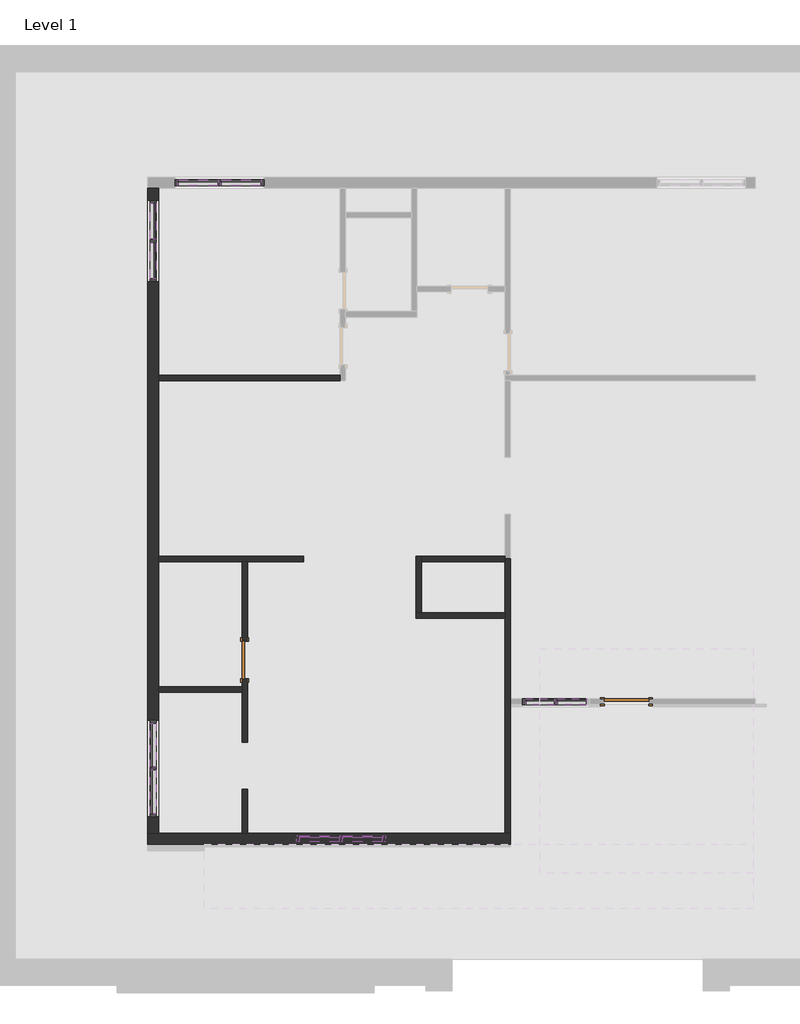
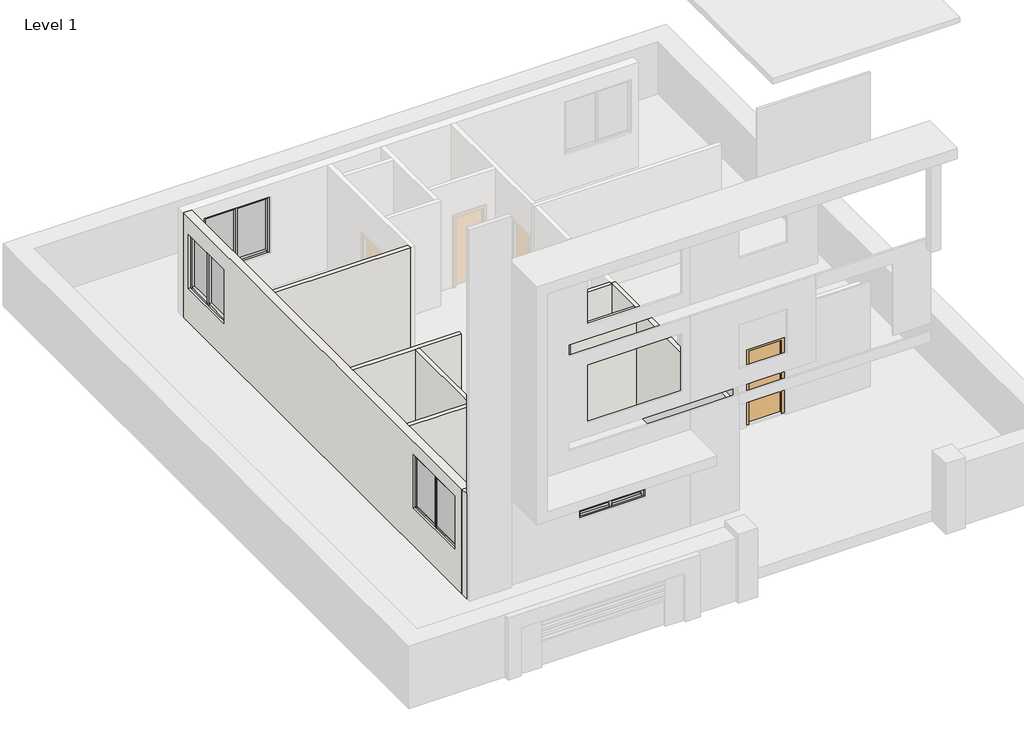
# One storey, part 1 of 2: 34 members, 11 walls, 10 plates, 2 doors.
"""IFC4 building model written with IfcOpenShell, lengths in millimetres."""

from ifc_helpers import new_model, si_unit, origin, origin_with_axes, place, context, project, spatial, polyline, outline, extrude, faceted_brep, transform, mapped, element, save
from components import door_f2b275c1, door_305aa2a5, member_c17f1be2, member_c9d9dd2f, member_dc22f6be, member_3a0a7659, member_087bde42, member_3d617b91, member_f1f71bde, member_fff76eb7, member_ea390ee7, member_e5d39754, member_6e88ea55, member_c4e92d7b, member_d19d9823, member_118fc41a, system_panel_glazed_f34af49f, system_panel_glazed_bfe2972e, system_panel_glazed_724d32f2, system_panel_glazed_a22ed96f, system_panel_glazed_9025697b

model = new_model("IFC4")

# Units and contexts
model_context = context("Model", 3, world=origin())
ifc_project = project(units=[si_unit("LENGTHUNIT", "METRE", prefix="MILLI")], contexts=[model_context])

# Site, building, storey
site = spatial("IfcSite", under=ifc_project)
building = spatial("IfcBuilding", under=site)
storey = spatial("IfcBuildingStorey", under=building, Name="Level 1", Elevation=0.0)

# Doors
placement = place(None, origin())
door_shape = door_f2b275c1(model_context)
element("IfcDoor", 1, ObjectType="Single-Flush : 30\" x 80\"", at=placement, inside=storey, context=model_context, shape_type="MappedRepresentation", body=[
    mapped(door_shape, transform((-16997.3695233, -10343.8252569, 0.0), x_axis=(0.0, -1.0, 0.0), y_axis=(1.0, 0.0, 0.0), z_axis=(0.0, 0.0, 1.0))),
])
door_2_shape = door_305aa2a5(model_context)
element("IfcDoor", 2, ObjectType="Single-Flush : 36\" x 84\"", at=placement, inside=storey, context=model_context, shape_type="MappedRepresentation", body=[
    mapped(door_2_shape, transform((-9148.7695233, -11201.0752569, 50.8), x_axis=(-1.0, 0.0, 0.0), y_axis=(0.0, -1.0, 0.0), z_axis=(0.0, 0.0, 1.0))),
])

# Members
member_shape = member_c17f1be2(model_context)
element("IfcMember", 3, ObjectType="Rectangular Mullion : 2.5\" x 5\" rectangular", at=placement, inside=storey, context=model_context, shape_type="MappedRepresentation", body=[
    mapped(member_shape, transform((-17543.4695233, -533.0752569, 2671.7497986), x_axis=(0.0, 0.0, 1.0), y_axis=(0.0, -1.0, 0.0), z_axis=(1.0, 0.0, 0.0))),
])
element("IfcMember", 4, ObjectType="Rectangular Mullion : 2.5\" x 5\" rectangular", at=placement, inside=storey, context=model_context, shape_type="MappedRepresentation", body=[
    mapped(member_shape, transform((-16660.8195233, -533.0752569, 2671.7497986), x_axis=(0.0, 0.0, 1.0), y_axis=(0.0, -1.0, 0.0), z_axis=(1.0, 0.0, 0.0))),
])
element("IfcMember", 5, ObjectType="Rectangular Mullion : 2.5\" x 5\" rectangular", at=placement, inside=storey, context=model_context, shape_type="MappedRepresentation", body=[
    mapped(member_shape, transform((-15047.9195233, -14020.4752569, 2510.0786282), x_axis=(0.0, 0.0, 1.0), y_axis=(0.0, -1.0, 0.0), z_axis=(1.0, 0.0, 0.0))),
])
element("IfcMember", 6, ObjectType="Rectangular Mullion : 2.5\" x 5\" rectangular", at=placement, inside=storey, context=model_context, shape_type="MappedRepresentation", body=[
    mapped(member_shape, transform((-14165.2695233, -14020.4752569, 2510.0786282), x_axis=(0.0, 0.0, 1.0), y_axis=(0.0, -1.0, 0.0), z_axis=(1.0, 0.0, 0.0))),
])
element("IfcMember", 7, ObjectType="Rectangular Mullion : 2.5\" x 5\" rectangular", at=placement, inside=storey, context=model_context, shape_type="MappedRepresentation", body=[
    mapped(member_shape, transform((-17479.9695233, -533.0752569, 1031.9306853), x_axis=(0.0, 0.0, -1.0), y_axis=(0.0, -1.0, 0.0), z_axis=(-1.0, 0.0, 0.0))),
])
element("IfcMember", 8, ObjectType="Rectangular Mullion : 2.5\" x 5\" rectangular", at=placement, inside=storey, context=model_context, shape_type="MappedRepresentation", body=[
    mapped(member_shape, transform((-18362.6195233, -533.0752569, 1031.9306853), x_axis=(0.0, 0.0, -1.0), y_axis=(0.0, -1.0, 0.0), z_axis=(-1.0, 0.0, 0.0))),
])
element("IfcMember", 9, ObjectType="Rectangular Mullion : 2.5\" x 5\" rectangular", at=placement, inside=storey, context=model_context, shape_type="MappedRepresentation", body=[
    mapped(member_shape, transform((-14984.4195233, -14020.4752569, 1270.940225), x_axis=(0.0, 0.0, -1.0), y_axis=(0.0, -1.0, 0.0), z_axis=(-1.0, 0.0, 0.0))),
])
element("IfcMember", 10, ObjectType="Rectangular Mullion : 2.5\" x 5\" rectangular", at=placement, inside=storey, context=model_context, shape_type="MappedRepresentation", body=[
    mapped(member_shape, transform((-15867.0695233, -14020.4752569, 1270.940225), x_axis=(0.0, 0.0, -1.0), y_axis=(0.0, -1.0, 0.0), z_axis=(-1.0, 0.0, 0.0))),
])
member_2_shape = member_c9d9dd2f(model_context)
element("IfcMember", 11, ObjectType="Rectangular Mullion : 2.5\" x 5\" rectangular", at=placement, inside=storey, context=model_context, shape_type="MappedRepresentation", body=[
    mapped(member_2_shape, transform((-17511.7195233, -533.0752569, 1031.9306853), x_axis=(1.0, 0.0, 0.0), y_axis=(0.0, -1.0, 0.0), z_axis=(0.0, 0.0, -1.0))),
])
member_3_shape = member_dc22f6be(model_context)
element("IfcMember", 12, ObjectType="Rectangular Mullion : 2.5\" x 5\" rectangular", at=placement, inside=storey, context=model_context, shape_type="MappedRepresentation", body=[
    mapped(member_3_shape, transform((-18426.1195233, -533.0752569, 2671.7497986), x_axis=(-1.0, 0.0, 0.0), y_axis=(0.0, -1.0, 0.0), z_axis=(0.0, 0.0, 1.0))),
])
element("IfcMember", 13, ObjectType="Rectangular Mullion : 2.5\" x 5\" rectangular", at=placement, inside=storey, context=model_context, shape_type="MappedRepresentation", body=[
    mapped(member_3_shape, transform((-16597.3195233, -533.0752569, 1031.9306853), x_axis=(1.0, 0.0, 0.0), y_axis=(0.0, -1.0, 0.0), z_axis=(0.0, 0.0, -1.0))),
])
member_4_shape = member_3a0a7659(model_context)
element("IfcMember", 14, ObjectType="Rectangular Mullion : 2.5\" x 5\" rectangular", at=placement, inside=storey, context=model_context, shape_type="MappedRepresentation", body=[
    mapped(member_4_shape, transform((-18883.3195233, -1701.4752569, 2563.3326118), x_axis=(0.0, 0.0, 1.0), y_axis=(-1.0, 0.0, 0.0), z_axis=(0.0, -1.0, 0.0))),
])
element("IfcMember", 15, ObjectType="Rectangular Mullion : 2.5\" x 5\" rectangular", at=placement, inside=storey, context=model_context, shape_type="MappedRepresentation", body=[
    mapped(member_4_shape, transform((-18883.3195233, -2507.9252569, 2563.3326118), x_axis=(0.0, 0.0, 1.0), y_axis=(-1.0, 0.0, 0.0), z_axis=(0.0, -1.0, 0.0))),
])
member_5_shape = member_087bde42(model_context)
element("IfcMember", 16, ObjectType="Rectangular Mullion : 2.5\" x 5\" rectangular", at=placement, inside=storey, context=model_context, shape_type="MappedRepresentation", body=[
    mapped(member_5_shape, transform((-18883.3195233, -1733.2252569, 993.8140067), x_axis=(0.0, -1.0, 0.0), y_axis=(-1.0, 0.0, 0.0), z_axis=(0.0, 0.0, -1.0))),
])
element("IfcMember", 17, ObjectType="Rectangular Mullion : 2.5\" x 5\" rectangular", at=placement, inside=storey, context=model_context, shape_type="MappedRepresentation", body=[
    mapped(member_4_shape, transform((-18883.3195233, -1764.9752569, 993.8140067), x_axis=(0.0, 0.0, -1.0), y_axis=(-1.0, 0.0, 0.0), z_axis=(0.0, 1.0, 0.0))),
])
element("IfcMember", 18, ObjectType="Rectangular Mullion : 2.5\" x 5\" rectangular", at=placement, inside=storey, context=model_context, shape_type="MappedRepresentation", body=[
    mapped(member_4_shape, transform((-18883.3195233, -958.5252569, 993.8140067), x_axis=(0.0, 0.0, -1.0), y_axis=(-1.0, 0.0, 0.0), z_axis=(0.0, 1.0, 0.0))),
])
member_6_shape = member_3d617b91(model_context)
element("IfcMember", 19, ObjectType="Rectangular Mullion : 2.5\" x 5\" rectangular", at=placement, inside=storey, context=model_context, shape_type="MappedRepresentation", body=[
    mapped(member_6_shape, transform((-18883.3195233, -2571.4252569, 993.8140067), x_axis=(0.0, -1.0, 0.0), y_axis=(-1.0, 0.0, 0.0), z_axis=(0.0, 0.0, -1.0))),
])
element("IfcMember", 20, ObjectType="Rectangular Mullion : 2.5\" x 5\" rectangular", at=placement, inside=storey, context=model_context, shape_type="MappedRepresentation", body=[
    mapped(member_6_shape, transform((-18883.3195233, -895.0252569, 2563.3326118), x_axis=(0.0, 1.0, 0.0), y_axis=(-1.0, 0.0, 0.0), z_axis=(0.0, 0.0, 1.0))),
])
member_7_shape = member_f1f71bde(model_context)
element("IfcMember", 21, ObjectType="Rectangular Mullion : 2.5\" x 5\" rectangular", at=placement, inside=storey, context=model_context, shape_type="MappedRepresentation", body=[
    mapped(member_7_shape, transform((-18883.3195233, -12604.4252569, 2650.6772749), x_axis=(0.0, 0.0, 1.0), y_axis=(1.0, 0.0, 0.0), z_axis=(0.0, 1.0, 0.0))),
])
element("IfcMember", 22, ObjectType="Rectangular Mullion : 2.5\" x 5\" rectangular", at=placement, inside=storey, context=model_context, shape_type="MappedRepresentation", body=[
    mapped(member_7_shape, transform((-18883.3195233, -11645.5752569, 2650.6772749), x_axis=(0.0, 0.0, 1.0), y_axis=(1.0, 0.0, 0.0), z_axis=(0.0, 1.0, 0.0))),
])
member_8_shape = member_fff76eb7(model_context)
element("IfcMember", 23, ObjectType="Rectangular Mullion : 2.5\" x 5\" rectangular", at=placement, inside=storey, context=model_context, shape_type="MappedRepresentation", body=[
    mapped(member_8_shape, transform((-18883.3195233, -12572.6752569, 1099.0426986), x_axis=(0.0, 1.0, 0.0), y_axis=(1.0, 0.0, 0.0), z_axis=(0.0, 0.0, -1.0))),
])
element("IfcMember", 24, ObjectType="Rectangular Mullion : 2.5\" x 5\" rectangular", at=placement, inside=storey, context=model_context, shape_type="MappedRepresentation", body=[
    mapped(member_7_shape, transform((-18883.3195233, -12540.9252569, 1099.0426986), x_axis=(0.0, 0.0, -1.0), y_axis=(1.0, 0.0, 0.0), z_axis=(0.0, -1.0, 0.0))),
])
element("IfcMember", 25, ObjectType="Rectangular Mullion : 2.5\" x 5\" rectangular", at=placement, inside=storey, context=model_context, shape_type="MappedRepresentation", body=[
    mapped(member_7_shape, transform((-18883.3195233, -13499.7752569, 1099.0426986), x_axis=(0.0, 0.0, -1.0), y_axis=(1.0, 0.0, 0.0), z_axis=(0.0, -1.0, 0.0))),
])
member_9_shape = member_ea390ee7(model_context)
element("IfcMember", 26, ObjectType="Rectangular Mullion : 2.5\" x 5\" rectangular", at=placement, inside=storey, context=model_context, shape_type="MappedRepresentation", body=[
    mapped(member_9_shape, transform((-18883.3195233, -13563.2752569, 2650.6772749), x_axis=(0.0, -1.0, 0.0), y_axis=(1.0, 0.0, 0.0), z_axis=(0.0, 0.0, 1.0))),
])
element("IfcMember", 27, ObjectType="Rectangular Mullion : 2.5\" x 5\" rectangular", at=placement, inside=storey, context=model_context, shape_type="MappedRepresentation", body=[
    mapped(member_9_shape, transform((-18883.3195233, -11582.0752569, 1099.0426986), x_axis=(0.0, 1.0, 0.0), y_axis=(1.0, 0.0, 0.0), z_axis=(0.0, 0.0, -1.0))),
])
member_10_shape = member_e5d39754(model_context)
element("IfcMember", 28, ObjectType="Rectangular Mullion : 2.5\" x 5\" rectangular", at=placement, inside=storey, context=model_context, shape_type="MappedRepresentation", body=[
    mapped(member_10_shape, transform((-10628.3195233, -11201.0752569, 2316.9077492), x_axis=(0.0, 0.0, 1.0), y_axis=(0.0, -1.0, 0.0), z_axis=(1.0, 0.0, 0.0))),
])
element("IfcMember", 29, ObjectType="Rectangular Mullion : 2.5\" x 5\" rectangular", at=placement, inside=storey, context=model_context, shape_type="MappedRepresentation", body=[
    mapped(member_10_shape, transform((-9974.2695233, -11201.0752569, 2316.9077492), x_axis=(0.0, 0.0, 1.0), y_axis=(0.0, -1.0, 0.0), z_axis=(1.0, 0.0, 0.0))),
])
member_11_shape = member_6e88ea55(model_context)
element("IfcMember", 30, ObjectType="Rectangular Mullion : 2.5\" x 5\" rectangular", at=placement, inside=storey, context=model_context, shape_type="MappedRepresentation", body=[
    mapped(member_11_shape, transform((-10596.5695233, -11201.0752569, 844.8572576), x_axis=(1.0, 0.0, 0.0), y_axis=(0.0, -1.0, 0.0), z_axis=(0.0, 0.0, -1.0))),
])
element("IfcMember", 31, ObjectType="Rectangular Mullion : 2.5\" x 5\" rectangular", at=placement, inside=storey, context=model_context, shape_type="MappedRepresentation", body=[
    mapped(member_10_shape, transform((-10564.8195233, -11201.0752569, 844.8572576), x_axis=(0.0, 0.0, -1.0), y_axis=(0.0, -1.0, 0.0), z_axis=(-1.0, 0.0, 0.0))),
])
element("IfcMember", 32, ObjectType="Rectangular Mullion : 2.5\" x 5\" rectangular", at=placement, inside=storey, context=model_context, shape_type="MappedRepresentation", body=[
    mapped(member_10_shape, transform((-11218.8695233, -11201.0752569, 844.8572576), x_axis=(0.0, 0.0, -1.0), y_axis=(0.0, -1.0, 0.0), z_axis=(-1.0, 0.0, 0.0))),
])
member_12_shape = member_c4e92d7b(model_context)
element("IfcMember", 33, ObjectType="Rectangular Mullion : 2.5\" x 5\" rectangular", at=placement, inside=storey, context=model_context, shape_type="MappedRepresentation", body=[
    mapped(member_12_shape, transform((-11282.3695233, -11201.0752569, 2316.9077492), x_axis=(-1.0, 0.0, 0.0), y_axis=(0.0, -1.0, 0.0), z_axis=(0.0, 0.0, 1.0))),
])
member_13_shape = member_d19d9823(model_context)
element("IfcMember", 34, ObjectType="Rectangular Mullion : 2.5\" x 5\" rectangular", at=placement, inside=storey, context=model_context, shape_type="MappedRepresentation", body=[
    mapped(member_13_shape, transform((-15016.1695233, -14020.4752569, 1270.940225), x_axis=(1.0, 0.0, 0.0), y_axis=(0.0, -1.0, 0.0), z_axis=(0.0, 0.0, -1.0))),
])
member_14_shape = member_118fc41a(model_context)
element("IfcMember", 35, ObjectType="Rectangular Mullion : 2.5\" x 5\" rectangular", at=placement, inside=storey, context=model_context, shape_type="MappedRepresentation", body=[
    mapped(member_14_shape, transform((-14101.7695233, -14020.4752569, 1270.940225), x_axis=(1.0, 0.0, 0.0), y_axis=(0.0, -1.0, 0.0), z_axis=(0.0, 0.0, -1.0))),
])
element("IfcMember", 36, ObjectType="Rectangular Mullion : 2.5\" x 5\" rectangular", at=placement, inside=storey, context=model_context, shape_type="MappedRepresentation", body=[
    mapped(member_14_shape, transform((-15930.5695233, -14020.4752569, 2510.0786282), x_axis=(-1.0, 0.0, 0.0), y_axis=(0.0, -1.0, 0.0), z_axis=(0.0, 0.0, 1.0))),
])

# Plates
system_panel_glazed_shape = system_panel_glazed_f34af49f(model_context)
element("IfcPlate", 37, ObjectType="System Panel : Glazed", at=placement, inside=storey, context=model_context, shape_type="MappedRepresentation", body=[
    mapped(system_panel_glazed_shape, transform((-17953.0445233, -533.0752569, 1095.4306853), x_axis=(1.0, 0.0, 0.0), y_axis=(0.0, 1.0, 0.0), z_axis=(0.0, 0.0, 1.0))),
])
element("IfcPlate", 38, ObjectType="System Panel : Glazed", at=placement, inside=storey, context=model_context, shape_type="MappedRepresentation", body=[
    mapped(system_panel_glazed_shape, transform((-17070.3945233, -533.0752569, 1095.4306853), x_axis=(1.0, 0.0, 0.0), y_axis=(0.0, 1.0, 0.0), z_axis=(0.0, 0.0, 1.0))),
])
system_panel_glazed_2_shape = system_panel_glazed_bfe2972e(model_context)
element("IfcPlate", 39, ObjectType="System Panel : Glazed", at=placement, inside=storey, context=model_context, shape_type="MappedRepresentation", body=[
    mapped(system_panel_glazed_2_shape, transform((-18883.3195233, -1330.0002569, 1057.3140067), x_axis=(0.0, -1.0, 0.0), y_axis=(1.0, 0.0, 0.0), z_axis=(0.0, 0.0, 1.0))),
])
element("IfcPlate", 40, ObjectType="System Panel : Glazed", at=placement, inside=storey, context=model_context, shape_type="MappedRepresentation", body=[
    mapped(system_panel_glazed_2_shape, transform((-18883.3195233, -2136.4502569, 1057.3140067), x_axis=(0.0, -1.0, 0.0), y_axis=(1.0, 0.0, 0.0), z_axis=(0.0, 0.0, 1.0))),
])
system_panel_glazed_3_shape = system_panel_glazed_724d32f2(model_context)
element("IfcPlate", 41, ObjectType="System Panel : Glazed", at=placement, inside=storey, context=model_context, shape_type="MappedRepresentation", body=[
    mapped(system_panel_glazed_3_shape, transform((-18883.3195233, -13052.1002569, 1162.5426986), x_axis=(0.0, 1.0, 0.0), y_axis=(-1.0, 0.0, 0.0), z_axis=(0.0, 0.0, 1.0))),
])
element("IfcPlate", 42, ObjectType="System Panel : Glazed", at=placement, inside=storey, context=model_context, shape_type="MappedRepresentation", body=[
    mapped(system_panel_glazed_3_shape, transform((-18883.3195233, -12093.2502569, 1162.5426986), x_axis=(0.0, 1.0, 0.0), y_axis=(-1.0, 0.0, 0.0), z_axis=(0.0, 0.0, 1.0))),
])
system_panel_glazed_4_shape = system_panel_glazed_a22ed96f(model_context)
element("IfcPlate", 43, ObjectType="System Panel : Glazed", at=placement, inside=storey, context=model_context, shape_type="MappedRepresentation", body=[
    mapped(system_panel_glazed_4_shape, transform((-10923.5945233, -11201.0752569, 908.3572576), x_axis=(1.0, 0.0, 0.0), y_axis=(0.0, 1.0, 0.0), z_axis=(0.0, 0.0, 1.0))),
])
element("IfcPlate", 44, ObjectType="System Panel : Glazed", at=placement, inside=storey, context=model_context, shape_type="MappedRepresentation", body=[
    mapped(system_panel_glazed_4_shape, transform((-10269.5445233, -11201.0752569, 908.3572576), x_axis=(1.0, 0.0, 0.0), y_axis=(0.0, 1.0, 0.0), z_axis=(0.0, 0.0, 1.0))),
])
system_panel_glazed_5_shape = system_panel_glazed_9025697b(model_context)
element("IfcPlate", 45, ObjectType="System Panel : Glazed", at=placement, inside=storey, context=model_context, shape_type="MappedRepresentation", body=[
    mapped(system_panel_glazed_5_shape, transform((-15457.4945233, -14020.4752569, 1334.440225), x_axis=(1.0, 0.0, 0.0), y_axis=(0.0, 1.0, 0.0), z_axis=(0.0, 0.0, 1.0))),
])
element("IfcPlate", 46, ObjectType="System Panel : Glazed", at=placement, inside=storey, context=model_context, shape_type="MappedRepresentation", body=[
    mapped(system_panel_glazed_5_shape, transform((-14574.8445233, -14020.4752569, 1334.440225), x_axis=(1.0, 0.0, 0.0), y_axis=(0.0, 1.0, 0.0), z_axis=(0.0, 0.0, 1.0))),
])

# Walls
element("IfcWall", 47, ObjectType="4.5\"", at=placement, inside=storey, context=model_context, shape_type="SweptSolid", body=[
    extrude(outline(polyline([(-18769.0195233, -4495.4752569), (-15035.2195233, -4495.4752569), (-15035.2195233, -4609.7752569), (-18769.0195233, -4609.7752569), (-18769.0195233, -4495.4752569)])), origin_with_axes(), (0.0, 0.0, 1.0), 3048.0),
])
element("IfcWall", 48, ObjectType="4.5\"", at=placement, inside=storey, context=model_context, shape_type="Brep", body=[
    faceted_brep([(-18769.0195233, -8324.5252569, 0.0), (-17054.5195233, -8324.5252569, 0.0), (-16940.2195233, -8324.5252569, 0.0), (-15784.5195233, -8324.5252569, 0.0), (-15784.5195233, -8324.5252569, 3048.0), (-16940.2195233, -8324.5252569, 3048.0), (-17054.5195233, -8324.5252569, 3048.0), (-18769.0195233, -8324.5252569, 3048.0), (-18769.0195233, -8210.2252569, 0.0), (-18769.0195233, -8210.2252569, 3048.0), (-15784.5195233, -8210.2252569, 3048.0), (-15784.5195233, -8210.2252569, 0.0)], [[[0, 1, 2, 3, 4, 5, 6, 7]], [[8, 9, 10, 11]], [[3, 2, 1, 0, 8, 11]], [[4, 3, 11, 10]], [[7, 6, 5, 4, 10, 9]], [[0, 7, 9, 8]]]),
])
element("IfcWall", 49, ObjectType="4.5\"", at=placement, inside=storey, context=model_context, shape_type="SweptSolid", body=[
    extrude(outline(polyline([(-16940.2195233, -13004.4752569), (-16940.2195233, -13906.1752569), (-17054.5195233, -13906.1752569), (-17054.5195233, -13004.4752569), (-16940.2195233, -13004.4752569)])), origin_with_axes(), (0.0, 0.0, 1.0), 3048.0),
])
element("IfcWall", 50, ObjectType="4.5\"", at=placement, inside=storey, context=model_context, shape_type="SweptSolid", body=[
    extrude(outline(polyline([(-18769.0195233, -10896.2752569), (-17054.5195233, -10896.2752569), (-17054.5195233, -11010.5752569), (-18769.0195233, -11010.5752569), (-18769.0195233, -10896.2752569)])), origin_with_axes(), (0.0, 0.0, 1.0), 3048.0),
])
element("IfcWall", 51, ObjectType="4.5\"", at=placement, inside=storey, context=model_context, shape_type="Brep", body=[
    faceted_brep([(-11644.3195233, -8267.3752569, 0.0), (-11644.3195233, -8324.5252569, 0.0), (-11644.3195233, -9372.2752569, 0.0), (-11644.3195233, -9486.5752569, 0.0), (-11644.3195233, -13906.1752569, 0.0), (-11644.3195233, -13906.1752569, 3048.0), (-11644.3195233, -9486.5752569, 3048.0), (-11644.3195233, -9372.2752569, 3048.0), (-11644.3195233, -8324.5252569, 3048.0), (-11644.3195233, -8267.3752569, 3048.0), (-11530.0195233, -8267.3752569, 0.0), (-11530.0195233, -8267.3752569, 3048.0), (-11530.0195233, -11143.9252569, 3048.0), (-11530.0195233, -11258.2252569, 3048.0), (-11530.0195233, -13906.1752569, 3048.0), (-11530.0195233, -13906.1752569, 0.0), (-11530.0195233, -11258.2252569, 0.0), (-11530.0195233, -11143.9252569, 0.0)], [[[0, 1, 2, 3, 4, 5, 6, 7, 8, 9]], [[10, 11, 12, 13, 14, 15, 16, 17]], [[4, 3, 2, 1, 0, 10, 17, 16, 15]], [[9, 8, 7, 6, 5, 14, 13, 12, 11]], [[0, 9, 11, 10]], [[5, 4, 15, 14]]]),
])
element("IfcWall", 52, ObjectType="4.5\"", at=placement, inside=storey, context=model_context, shape_type="Brep", body=[
    faceted_brep([(-11644.3195233, -9372.2752569, 0.0), (-13358.8195233, -9372.2752569, 0.0), (-13473.1195233, -9372.2752569, 0.0), (-13473.1195233, -9372.2752569, 3048.0), (-13358.8195233, -9372.2752569, 3048.0), (-11644.3195233, -9372.2752569, 3048.0), (-11644.3195233, -9486.5752569, 0.0), (-11644.3195233, -9486.5752569, 3048.0), (-13473.1195233, -9486.5752569, 3048.0), (-13473.1195233, -9486.5752569, 0.0)], [[[0, 1, 2, 3, 4, 5]], [[6, 7, 8, 9]], [[2, 1, 0, 6, 9]], [[5, 4, 3, 8, 7]], [[0, 5, 7, 6]], [[3, 2, 9, 8]]]),
])
element("IfcWall", 53, ObjectType="4.5\"", at=placement, inside=storey, context=model_context, shape_type="Brep", body=[
    faceted_brep([(-13358.8195233, -9372.2752569, 0.0), (-13358.8195233, -8324.5252569, 0.0), (-13358.8195233, -8210.2252569, 0.0), (-13358.8195233, -8210.2252569, 3048.0), (-13358.8195233, -8324.5252569, 3048.0), (-13358.8195233, -9372.2752569, 3048.0), (-13473.1195233, -9372.2752569, 0.0), (-13473.1195233, -9372.2752569, 3048.0), (-13473.1195233, -8210.2252569, 3048.0), (-13473.1195233, -8210.2252569, 0.0)], [[[0, 1, 2, 3, 4, 5]], [[6, 7, 8, 9]], [[2, 1, 0, 6, 9]], [[5, 4, 3, 8, 7]], [[0, 5, 7, 6]], [[3, 2, 9, 8]]]),
])
element("IfcWall", 54, ObjectType="4.5\"", at=placement, inside=storey, context=model_context, shape_type="Brep", body=[
    faceted_brep([(-16940.2195233, -12039.2752569, 0.0), (-16940.2195233, -10724.8252569, 0.0), (-16940.2195233, -10724.8252569, 2032.0), (-16940.2195233, -9962.8252569, 2032.0), (-16940.2195233, -9962.8252569, 0.0), (-16940.2195233, -8324.5252569, 0.0), (-16940.2195233, -8324.5252569, 3048.0), (-16940.2195233, -12039.2752569, 3048.0), (-17054.5195233, -10724.8252569, 2032.0), (-17054.5195233, -10724.8252569, 0.0), (-17054.5195233, -10896.2752569, 0.0), (-17054.5195233, -11010.5752569, 0.0), (-17054.5195233, -12039.2752569, 0.0), (-17054.5195233, -12039.2752569, 3048.0), (-17054.5195233, -11010.5752569, 3048.0), (-17054.5195233, -10896.2752569, 3048.0), (-17054.5195233, -8324.5252569, 3048.0), (-17054.5195233, -8324.5252569, 0.0), (-17054.5195233, -9962.8252569, 0.0), (-17054.5195233, -9962.8252569, 2032.0)], [[[0, 1, 2, 3, 4, 5, 6, 7]], [[8, 9, 10, 11, 12, 13, 14, 15, 16, 17, 18, 19]], [[18, 17, 5, 4]], [[12, 11, 10, 9, 1, 0]], [[7, 6, 16, 15, 14, 13]], [[0, 7, 13, 12]], [[6, 5, 17, 16]], [[4, 3, 19, 18]], [[3, 2, 8, 19]], [[2, 1, 9, 8]]]),
])
element("IfcWall", 55, ObjectType="4.5\"", at=placement, inside=storey, context=model_context, shape_type="Brep", body=[
    faceted_brep([(-13358.8195233, -8324.5252569, 0.0), (-11644.3195233, -8324.5252569, 0.0), (-11644.3195233, -8324.5252569, 3048.0), (-13358.8195233, -8324.5252569, 3048.0), (-13358.8195233, -8210.2252569, 0.0), (-13358.8195233, -8210.2252569, 3048.0), (-11644.3195233, -8210.2252569, 3048.0), (-11644.3195233, -8210.2252569, 0.0), (-11644.3195233, -8267.3752569, 0.0), (-11644.3195233, -8267.3752569, 3048.0)], [[[0, 1, 2, 3]], [[4, 5, 6, 7]], [[1, 0, 4, 7, 8]], [[3, 2, 9, 6, 5]], [[2, 1, 8, 7, 6, 9]], [[0, 3, 5, 4]]]),
])
element("IfcWall", 56, ObjectType="9\"", at=placement, inside=storey, context=model_context, shape_type="Brep", body=[
    faceted_brep([(-18997.6195233, -14134.7752569, 0.0), (-11530.0195233, -14134.7752569, 0.0), (-11530.0195233, -14134.7752569, 3048.0), (-18997.6195233, -14134.7752569, 3048.0), (-15930.5695233, -14134.7752569, 1270.940225), (-15930.5695233, -14134.7752569, 2510.0786282), (-14101.7695233, -14134.7752569, 2510.0786282), (-14101.7695233, -14134.7752569, 1270.940225), (-11530.0195233, -13906.1752569, 0.0), (-11644.3195233, -13906.1752569, 0.0), (-16940.2195233, -13906.1752569, 0.0), (-17054.5195233, -13906.1752569, 0.0), (-18769.0195233, -13906.1752569, 0.0), (-18997.6195233, -13906.1752569, 0.0), (-18997.6195233, -13906.1752569, 3048.0), (-18769.0195233, -13906.1752569, 3048.0), (-17054.5195233, -13906.1752569, 3048.0), (-16940.2195233, -13906.1752569, 3048.0), (-11644.3195233, -13906.1752569, 3048.0), (-11530.0195233, -13906.1752569, 3048.0), (-15930.5695233, -13906.1752569, 2510.0786282), (-15930.5695233, -13906.1752569, 1270.940225), (-14101.7695233, -13906.1752569, 1270.940225), (-14101.7695233, -13906.1752569, 2510.0786282)], [[[0, 1, 2, 3], [4, 5, 6, 7]], [[8, 9, 10, 11, 12, 13, 14, 15, 16, 17, 18, 19], [20, 21, 22, 23]], [[1, 0, 13, 12, 11, 10, 9, 8]], [[2, 1, 8, 19]], [[3, 2, 19, 18, 17, 16, 15, 14]], [[0, 3, 14, 13]], [[4, 21, 20, 5]], [[5, 20, 23, 6]], [[6, 23, 22, 7]], [[21, 4, 7, 22]]]),
])
element("IfcWall", 57, ObjectType="9\"", at=placement, inside=storey, context=model_context, shape_type="Brep", body=[
    faceted_brep([(-18997.6195233, -647.3752569, 0.0), (-18997.6195233, -13906.1752569, 0.0), (-18997.6195233, -13906.1752569, 3048.0), (-18997.6195233, -647.3752569, 3048.0), (-18997.6195233, -895.0252569, 993.8140067), (-18997.6195233, -895.0252569, 2563.3326118), (-18997.6195233, -2571.4252569, 2563.3326118), (-18997.6195233, -2571.4252569, 993.8140067), (-18997.6195233, -13563.2752569, 2650.6772749), (-18997.6195233, -13563.2752569, 1099.0426986), (-18997.6195233, -11582.0752569, 1099.0426986), (-18997.6195233, -11582.0752569, 2650.6772749), (-18769.0195233, -13906.1752569, 0.0), (-18769.0195233, -11010.5752569, 0.0), (-18769.0195233, -10896.2752569, 0.0), (-18769.0195233, -8324.5252569, 0.0), (-18769.0195233, -8210.2252569, 0.0), (-18769.0195233, -4609.7752569, 0.0), (-18769.0195233, -4495.4752569, 0.0), (-18769.0195233, -647.3752569, 0.0), (-18769.0195233, -647.3752569, 3048.0), (-18769.0195233, -4495.4752569, 3048.0), (-18769.0195233, -4609.7752569, 3048.0), (-18769.0195233, -8210.2252569, 3048.0), (-18769.0195233, -8324.5252569, 3048.0), (-18769.0195233, -10896.2752569, 3048.0), (-18769.0195233, -11010.5752569, 3048.0), (-18769.0195233, -13906.1752569, 3048.0), (-18769.0195233, -895.0252569, 2563.3326118), (-18769.0195233, -895.0252569, 993.8140067), (-18769.0195233, -2571.4252569, 993.8140067), (-18769.0195233, -2571.4252569, 2563.3326118), (-18769.0195233, -13563.2752569, 1099.0426986), (-18769.0195233, -13563.2752569, 2650.6772749), (-18769.0195233, -11582.0752569, 2650.6772749), (-18769.0195233, -11582.0752569, 1099.0426986)], [[[0, 1, 2, 3], [4, 5, 6, 7], [8, 9, 10, 11]], [[12, 13, 14, 15, 16, 17, 18, 19, 20, 21, 22, 23, 24, 25, 26, 27], [28, 29, 30, 31], [32, 33, 34, 35]], [[1, 0, 19, 18, 17, 16, 15, 14, 13, 12]], [[3, 2, 27, 26, 25, 24, 23, 22, 21, 20]], [[2, 1, 12, 27]], [[0, 3, 20, 19]], [[4, 29, 28, 5]], [[5, 28, 31, 6]], [[6, 31, 30, 7]], [[29, 4, 7, 30]], [[32, 9, 8, 33]], [[33, 8, 11, 34]], [[10, 35, 34, 11]], [[9, 32, 35, 10]]]),
])

save(model, "model.ifc")

# Revit data of these elements
# Type "Single-Flush : 30\" x 80\""
#   Type Mark = "5"
#   Construction Type Id = "MDOOR"
#   Assembly Code = "C1020"
#   Analytic Construction = "Metal"
#   Thickness = 0' - 2"
#   Heat Transfer Coefficient (U) = 0.651978 BTU/(h·ft²·°F)
#   Height = 6' - 8"
#   Trim Projection Ext = 0' - 1"
#   Trim Projection Int = 0' - 1"
#   Trim Width = 0' - 3"
#   Width = 2' - 6"
#   Define Thermal Properties by = 1
#   Define Thermal Properties by = 1
#   Door Material = Door - Panel
#   Frame Material = Door - Frame
#   Visual Light Transmittance = 0
#   Solar Heat Gain Coefficient = 0
#   Function = (empty or 0)
#   Wall Closure = (empty or 0)
# Type "Single-Flush : 36\" x 84\""
#   Type Mark = "1"
#   Construction Type Id = "MDOOR"
#   Assembly Code = "C1020"
#   Analytic Construction = "Metal"
#   Thickness = 0' - 2"
#   Heat Transfer Coefficient (U) = 0.651978 BTU/(h·ft²·°F)
#   Height = 7' - 0"
#   Trim Projection Ext = 0' - 1"
#   Trim Projection Int = 0' - 1"
#   Trim Width = 0' - 3"
#   Width = 3' - 0"
#   Define Thermal Properties by = 1
#   Define Thermal Properties by = 1
#   Door Material = Door - Panel
#   Frame Material = Door - Frame
#   Visual Light Transmittance = 0
#   Solar Heat Gain Coefficient = 0
#   Function = (empty or 0)
#   Wall Closure = (empty or 0)
# Type "Rectangular Mullion : 2.5\" x 5\" rectangular"
#   built-in parameter 1007304 = 0.416667 (stored number, unit not read)
#   built-in parameter 1007301 = 0.104167 (stored number, unit not read)
#   built-in parameter 1007300 = 0.104167 (stored number, unit not read)
# Type "System Panel : Glazed"
#   Construction Type Id = "GSP4R"
#   Analytic Construction = "1/8 in Pilkington single glazing"
#   Visual Light Transmittance = 0.9
#   Solar Heat Gain Coefficient = 0.86
#   Heat Transfer Coefficient (U) = 1.18115 BTU/(h·ft²·°F)
#   Define Thermal Properties by = 1
# Type "4.5\""
#   Assembly Code = "B2010"
#   Layers, outside or top first: 0' - 4 1/2" no material (function 1)
# Type "9\""
#   Assembly Code = "B2010"
#   Layers, outside or top first: 0' - 9" no material (function 1)
# Element 1 (IfcDoor, "Single-Flush : 30\" x 80\"")
#   Phase Created = New Construction
#   Materials on its faces: "Door - Frame", "Door - Panel"
# Element 2 (IfcDoor, "Single-Flush : 36\" x 84\"")
#   Phase Created = New Construction
#   Materials on its faces: "Door - Frame", "Door - Panel"
# Elements 3, 4, 5, 6, 7, 8, 9, 10, 11, 12, 13, 14, 15, 16, 17, 18, 19, 20, 21, 22, 23, 24, 25, 26, 27, 28, 29, 30, 31, 32, 33, 34, 35, 36 (IfcMember, "Rectangular Mullion : 2.5\" x 5\" rectangular")
#   Phase Created = New Construction
#   Materials on its faces: "Aluminum"
# Elements 37, 38, 39, 40, 41, 42, 43, 44, 45, 46 (IfcPlate, "System Panel : Glazed")
#   Phase Created = New Construction
#   Materials on its faces: "Glass"
# Elements 47, 48, 49, 50, 51, 52, 53, 54, 55 (IfcWall, "4.5\"")
#   Top Offset = 0' - 0"
#   Base Offset = 0' - 0"
#   Unconnected Height = 10' - 0"
#   wall height = 10' - 0"
#   Phase Created = New Construction
#   Base Constraint = Level 1
#   Materials on its faces: "Default Wall"
# Elements 56, 57 (IfcWall, "9\"")
#   Top Offset = 0' - 0"
#   Base Offset = 0' - 0"
#   Unconnected Height = 10' - 0"
#   wall height = 10' - 0"
#   Phase Created = New Construction
#   Base Constraint = Level 1
#   Materials on its faces: "Default Wall"
# Materials
#   "Door - Panel": class "Wood", colour RGB 210 159 95, transparency 0, Cost = 0
#   "Door - Frame": colour RGB 118 70 51, transparency 0, Cost = 0
#   "Aluminum": class "Metal", colour RGB 247 247 247, transparency 0, Description = "Aluminum 6061", Cost = 0
#   "Glass": class "Glass", colour RGB 0 128 192, transparency 0.75, Description = "Soda Lime Glass", Cost = 0
#   "Default Wall": colour RGB 128 128 128, transparency 0, Cost = 0
